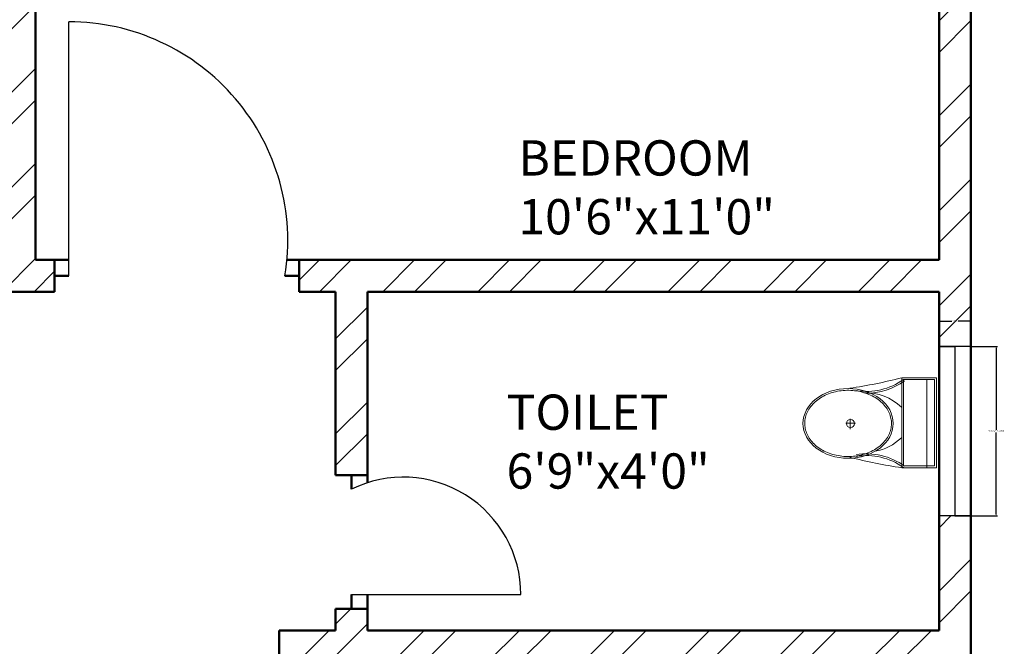
# Model space of a CAD drawing. Units: inches. Extents: x 1901 to 2863, y 888 to 2433.
# Tile 40 of 91: x 2618 to 2758, y 1474 to 1563. Entities that reach past the tile are written whole.
import ezdxf

# ---------------------------------------------------------------- set-up
doc = ezdxf.new("R2010")
doc.units = ezdxf.units.IN
for name, color, linetype, lineweight in [('A-ANNO-DIMS', 2, 'Continuous', 18), ('A-AREA-IDEN', 7, 'Continuous', 18), ('A-DOOR', 4, 'Continuous', 25), ('A-FLOR-FIXT', 9, 'Continuous', 18), ('A-GLAZ', 3, 'Continuous', 25), ('A-WALL', 7, 'Continuous', 50), ('A-WALL-PATT', 8, 'Continuous', 13)]:
    doc.layers.add(name, color=color, linetype=linetype, lineweight=lineweight)
doc.styles.get("Standard").update_dxf_attribs({"font": 'arial.ttf'})
doc.dimstyles.get("Standard").update_dxf_attribs({"dimtxt": 0.18, "dimasz": 0.18, "dimexe": 0.18, "dimexo": 0.0625, "dimgap": 0.09, "dimtad": 0, "dimtih": 1, "dimtoh": 1, "dimdec": 4, "dimzin": 0, "dimdsep": 46, "dimtxsty": 'Standard', "dimcen": 0.09, "dimadec": 0, "dimazin": 0, "dimtfac": 1, "dimtdec": 4, "dimtofl": 0, "dimtmove": 0, "dimatfit": 3, "dimfxl": 1, "dimtolj": 1, "dimtzin": 0, "dimarcsym": 0})

# ---------------------------------------------------------------- blocks, each defined once
blk = doc.blocks.new('A$C31115884')
for p, q in [((257.5, 466.4), (257.5, 523.2)), ((283.1, 497.7), (223.4, 497.7)), ((0, 200), (0, 0)), ((520, 200), (0, 200)), ((10, 190), (10, 10)), ((510, 190), (10, 190)), ((510, 10), (510, 190)), ((520, 0), (520, 200)), ((510, 54.5), (0, 54.5)), ((10, 10), (510, 10)), ((0, 0), (520, 0))]:
    blk.add_line(p, q)
blk.add_circle((255.6, 496.4), 23.6)
for centre, radius, start, end in [((2777.7, -204.6), 2807, 165.4549, 171.7133), ((-294.5, 403.3), 364.7, 324.2091, 9.3499), ((-294.5, 403.3), 374.7, 324.2091, 9.3499), ((805.8, 403.3), 364.7, 170.6501, 215.7909), ((3237, 905), 2807, 188.2867, 194.5451), ((139.5, 406.2), 293.5, 315.8436, 2.6563), ((805.8, 403.3), 374.7, 179.2036, 215.7909), ((383.6, 406.2), 293.5, 190.2774, 224.1564)]:
    blk.add_arc(centre, radius, start, end)
blk.add_ellipse((256.2, 509.9), major_axis=(0, -260.7), ratio=0.772727)
blk.add_open_spline([(256.2, 259.2), (263.1, 259.2), (270, 259.7), (287.8, 262.3), (298.7, 265.1), (319.9, 273.1), (330.2, 278.4), (350.1, 291.1), (359.7, 298.7), (377.7, 315.9), (386.2, 325.5), (401.7, 346.6), (408.8, 358.1), (421.3, 382.5), (426.8, 395.5), (435.9, 422.4), (439.5, 436.4), (444.8, 465.1), (446.5, 479.7), (447.9, 509.2), (447.6, 524), (445, 553.3), (442.7, 567.8), (436.3, 596), (432.1, 609.7), (421.9, 636), (416, 648.6), (402.5, 672.1), (395, 683), (378.6, 703), (369.8, 712.1), (351.1, 728), (341.3, 734.8), (320.9, 746.2), (310.4, 750.7), (288.9, 757.3), (278, 759.4), (256, 761), (245, 760.6), (223.1, 757.2), (212.3, 754.3), (191.1, 746.1), (180.8, 740.7), (160.9, 727.8), (151.4, 720.1), (133.5, 702.7), (125.1, 693), (109.6, 671.7), (102.6, 660.2), (90.2, 635.7), (84.9, 622.7), (76, 595.6), (72.4, 581.6), (67.2, 552.9), (65.6, 538.2), (64.4, 508.8), (64.8, 494), (67.5, 464.7), (69.9, 450.2), (76.6, 422), (80.8, 408.3), (91.1, 382.2), (97.2, 369.7), (110.8, 346.3), (118.4, 335.4), (134.8, 315.6), (143.7, 306.7), (162.4, 290.9), (172.3, 284.2), (192.8, 273), (203.3, 268.6), (224.8, 262.2), (235.8, 260.2), (249.9, 259.3), (253, 259.2), (256.2, 259.2)], degree=3, knots=[0, 0, 0, 0, 0.110105, 0.110105, 0.285049, 0.285049, 0.459994, 0.459994, 0.634938, 0.634938, 0.809882, 0.809882, 0.984827, 0.984827, 1.159771, 1.159771, 1.334715, 1.334715, 1.50966, 1.50966, 1.684604, 1.684604, 1.859549, 1.859549, 2.034493, 2.034493, 2.209437, 2.209437, 2.384382, 2.384382, 2.559326, 2.559326, 2.73427, 2.73427, 2.909215, 2.909215, 3.084159, 3.084159, 3.259103, 3.259103, 3.434048, 3.434048, 3.608992, 3.608992, 3.783936, 3.783936, 3.958881, 3.958881, 4.133825, 4.133825, 4.30877, 4.30877, 4.483714, 4.483714, 4.658658, 4.658658, 4.833603, 4.833603, 5.008547, 5.008547, 5.183491, 5.183491, 5.358436, 5.358436, 5.53338, 5.53338, 5.708324, 5.708324, 5.883269, 5.883269, 6.058213, 6.058213, 6.233158, 6.233158, 6.283185, 6.283185, 6.283185, 6.283185])
blk = doc.blocks.new('WIN-24')
for p, q in [((0, 4.5), (0, 0)), ((24, 2.25), (24, 4.5)), ((24, 4.5), (24, 0)), ((0, 0), (0, 2.25)), ((0, 2.25), (24, 2.25))]:
    blk.add_line(p, q)
blk = doc.blocks.new('*D23')
at = {"layer": 'A-ANNO-DIMS', "color": 0, "lineweight": -2, "transparency": 16777216}
for p, q in [((2752.99, 1516.88), (2756.71, 1516.88)), ((2756.53, 1516.7), (2756.53, 1505.06)), ((2756.53, 1493.06), (2756.53, 1504.7)), ((2752.99, 1492.88), (2756.71, 1492.88))]:
    blk.add_line(p, q, dxfattribs=at)
at = {"layer": 'A-ANNO-DIMS', "color": 0, "transparency": 16777216}
for points in [[(2756.5, 1516.7), (2756.56, 1516.7), (2756.53, 1516.88)], [(2756.5, 1493.06), (2756.56, 1493.06), (2756.53, 1492.88)]]:
    blk.add_solid(points, dxfattribs=at)
at = {"layer": 'Defpoints', "color": 0, "transparency": 16777216}
for p in [(2752.93, 1516.88), (2752.93, 1492.88), (2756.53, 1492.88)]:
    blk.add_point(p, dxfattribs=at)
at = {"layer": 'A-ANNO-DIMS', "color": 0, "transparency": 16777216, "insert": (2756.53, 1504.88), "char_height": 0.18, "attachment_point": 5}
blk.add_mtext('\\A1;WINDOW W3 24 TYP.', dxfattribs=at)
blk = doc.blocks.new('*D24')
at = {"layer": 'A-ANNO-DIMS', "color": 0, "lineweight": -2, "transparency": 16777216}
for p, q in [((2748.43, 1516.94), (2748.43, 1520.66)), ((2748.61, 1520.48), (2750.22, 1520.48)), ((2752.75, 1520.48), (2751.13, 1520.48)), ((2752.93, 1516.94), (2752.93, 1520.66))]:
    blk.add_line(p, q, dxfattribs=at)
at = {"layer": 'A-ANNO-DIMS', "color": 0, "transparency": 16777216}
for points in [[(2748.61, 1520.51), (2748.61, 1520.45), (2748.43, 1520.48)], [(2752.75, 1520.51), (2752.75, 1520.45), (2752.93, 1520.48)]]:
    blk.add_solid(points, dxfattribs=at)
at = {"layer": 'Defpoints', "color": 0, "transparency": 16777216}
for p in [(2752.93, 1520.48), (2748.43, 1516.88), (2752.93, 1516.88)]:
    blk.add_point(p, dxfattribs=at)
at = {"layer": 'A-ANNO-DIMS', "color": 0, "transparency": 16777216, "insert": (2750.68, 1520.48), "char_height": 0.18, "attachment_point": 5}
blk.add_mtext('\\A1;5 TYP.', dxfattribs=at)

msp = doc.modelspace()

# ---------------------------------------------------------------- hatches: boundary and pattern name
at = {"layer": 'A-WALL-PATT'}
h = msp.add_hatch(dxfattribs=at)
h.set_pattern_fill('ANSI32', color=256)
h.paths.add_polyline_path([(2192.5, 2274.13), (2141.26, 2274.13), (2141.26, 2269.63), (2192.5, 2269.63)])
h.paths.add_polyline_path([(2259.93, 2274.13), (2216.5, 2274.13), (2216.5, 2269.63), (2255.43, 2269.63), (2255.43, 2214.63), (2250.81, 2214.63), (2250.81, 2210.13), (2259.93, 2210.13), (2259.93, 2215.13), (2271.76, 2215.13), (2271.76, 2217.38), (2271.76, 2219.63), (2259.93, 2219.63)])
h.paths.add_polyline_path([(2171.43, 2269.63), (2166.93, 2269.63), (2166.93, 2219.63), (2121.24, 2219.63), (2121.24, 2215.13), (2166.93, 2215.13), (2166.93, 2083.13), (2161.81, 2083.13), (2161.81, 2078.63), (2171.43, 2078.63), (2177, 2078.63), (2177, 2080.88), (2177, 2083.13), (2171.43, 2083.13), (2171.43, 2210.13), (2230.91, 2210.13), (2230.91, 2212.38), (2230.91, 2214.63), (2171.43, 2214.63)])
h.paths.add_polyline_path([(2117.26, 2274.13), (2089.43, 2274.13), (2089.43, 2219.63), (2081.14, 2219.63), (2081.14, 2215.13), (2089.43, 2215.13), (2098, 2215.13), (2098, 2217.38), (2098, 2219.63), (2093.93, 2219.63), (2093.93, 2269.63), (2117.26, 2269.63), (2117.26, 2271.88)])
h.paths.add_polyline_path([(2343.43, 2219.63), (2329.29, 2219.63), (2329.29, 2215.13), (2338.93, 2215.13), (2338.93, 2184.74), (2343.43, 2184.74)])
h.paths.add_polyline_path([(2338.93, 2083.13), (2329.29, 2083.13), (2208.97, 2083.13), (2208.97, 2078.63), (2338.93, 2078.63)])
h.paths.add_polyline_path([(2343.43, 2136.74), (2338.93, 2136.74), (2338.93, 1872.63), (2343.43, 1872.63)])
h.paths.add_polyline_path([(2343.43, 1863.63), (2397.68, 1863.63), (2397.68, 1821.63), (2384.14, 1821.63), (2384.14, 1812.63), (2418.33, 1812.63), (2418.33, 1817.13), (2418.33, 1821.63), (2406.68, 1821.63), (2406.68, 1863.63), (2459.5, 1863.63), (2459.5, 1821.63), (2447.14, 1821.63), (2447.14, 1812.63), (2459.5, 1812.63), (2468.5, 1812.63), (2468.5, 1872.63), (2394.43, 1872.63), (2334.43, 1872.63), (2334.43, 1812.63), (2343.43, 1812.63), (2353.25, 1812.63), (2353.25, 1821.63), (2343.43, 1821.63)])
h.paths.add_polyline_path([(2510.01, 1872.63), (2468.5, 1872.63), (2468.5, 1868.13), (2510.01, 1868.13)])
h.paths.add_polyline_path([(2514.01, 1817.13), (2468.5, 1817.13), (2468.5, 1812.63), (2482.11, 1812.63), (2482.11, 1800.61), (2486.61, 1800.61), (2486.61, 1812.63), (2514.01, 1812.63)])
h.paths.add_polyline_path([(2299.25, 1814.88), (2299.25, 1817.13), (2295.93, 1817.13), (2295.93, 1854.17), (2293.68, 1854.17), (2291.43, 1854.17), (2291.43, 1817.13), (2266.11, 1817.13), (2266.11, 1812.63), (2299.25, 1812.63)])
h.paths.add_polyline_path([(2218.11, 1817.13), (2206.46, 1817.13), (2171.43, 1817.13), (2171.43, 1949.13), (2190.1, 1949.13), (2190.1, 1953.63), (2163.47, 1953.63), (2163.47, 1949.13), (2166.93, 1949.13), (2166.93, 1817.13), (2114.3, 1817.13), (2114.3, 1812.63), (2218.11, 1812.63)])
h.paths.add_polyline_path([(2029.43, 1970.92), (2024.93, 1970.92), (2024.93, 1912.72), (2029.43, 1912.72)])
h.paths.add_polyline_path([(2132.3, 1953.63), (2113.93, 1953.63), (2113.93, 1975.89), (2111.68, 1975.89), (2109.43, 1975.89), (2109.43, 1953.63), (2029.43, 1953.63), (2029.43, 1949.13), (2132.3, 1949.13)])
h.paths.add_polyline_path([(2029.43, 1853.61), (2029.31, 1853.61), (2029.31, 1853.61), (2029.43, 1853.61), (2029.43, 1864.72), (2024.93, 1864.72), (2024.93, 1812.63), (2066.3, 1812.63), (2066.3, 1814.88), (2066.3, 1817.13), (2029.43, 1817.13)])
h.paths.add_polyline_path([(2122.93, 2010.09), (2120.68, 2010.09), (2118.43, 2010.09), (2118.43, 2006.13), (2029.43, 2006.13), (2029.43, 2001.63), (2109.43, 2001.63), (2109.43, 1998.04), (2113.93, 1998.04), (2113.93, 2001.63), (2122.93, 2001.63)])
h.paths.add_polyline_path([(2029.43, 2031.38), (2024.93, 2031.38), (2024.93, 1994.92), (2027.18, 1994.92), (2029.43, 1994.92)])
h.paths.add_polyline_path([(2029.43, 2136.74), (2024.93, 2136.74), (2024.93, 2067.38), (2027.18, 2067.38), (2029.43, 2067.38)])
h.paths.add_polyline_path([(2125.62, 2083.13), (2029.43, 2083.13), (2029.43, 2078.63), (2118.43, 2078.63), (2118.43, 2030.71), (2122.93, 2030.71), (2122.93, 2078.63), (2125.62, 2078.63)])
h.paths.add_polyline_path([(2029.43, 2215.13), (2040.47, 2215.13), (2040.47, 2217.38), (2040.47, 2219.63), (2024.93, 2219.63), (2024.93, 2184.74), (2029.43, 2184.74), (2029.43, 2187.78)])
h.paths.add_polyline_path([(2686.43, 2274.13), (2659.28, 2274.13), (2659.28, 2269.63), (2681.93, 2269.63), (2681.93, 2219.63), (2676.82, 2219.63), (2676.82, 2215.13), (2681.93, 2215.13), (2697.01, 2215.13), (2697.01, 2217.38), (2697.01, 2219.63), (2686.43, 2219.63)])
h.paths.add_polyline_path([(2609.93, 2269.63), (2635.28, 2269.63), (2635.28, 2274.13), (2571.43, 2274.13), (2571.43, 2269.63), (2605.43, 2269.63), (2605.43, 2214.63), (2549.1, 2214.63), (2549.1, 2210.13), (2605.43, 2210.13), (2605.43, 2083.13), (2601.01, 2083.13), (2601.01, 2080.88), (2601.01, 2078.63), (2609.93, 2078.63), (2616.16, 2078.63), (2616.16, 2080.88), (2616.16, 2083.13), (2609.93, 2083.13), (2609.93, 2215.13), (2651.46, 2215.13), (2651.46, 2217.38), (2651.46, 2219.63), (2609.93, 2219.63)])
h.paths.add_polyline_path([(2521.43, 2269.63), (2547.43, 2269.63), (2547.43, 2271.88), (2547.43, 2274.13), (2516.93, 2274.13), (2516.93, 2219.63), (2506.41, 2219.63), (2506.41, 2215.13), (2516.93, 2215.13), (2516.93, 2210.13), (2525.4, 2210.13), (2525.4, 2212.38), (2525.4, 2214.63), (2521.43, 2214.63)])
h.paths.add_polyline_path([(2456.01, 2219.63), (2439.43, 2219.63), (2439.43, 2187.89), (2443.93, 2187.89), (2443.93, 2215.13), (2456.01, 2215.13)])
h.paths.add_polyline_path([(2752.93, 2219.63), (2739.48, 2219.63), (2739.48, 2215.13), (2748.43, 2215.13), (2748.43, 2187.89), (2752.93, 2187.89)])
h.paths.add_polyline_path([(2752.93, 2139.89), (2748.43, 2139.89), (2748.43, 2083.13), (2648.42, 2083.13), (2648.42, 2078.63), (2654.93, 2078.63), (2654.93, 2039.44), (2659.43, 2039.44), (2659.43, 2078.63), (2748.43, 2078.63), (2748.43, 2063.43), (2752.93, 2063.43)])
h.paths.add_polyline_path([(2752.93, 2010.63), (2659.43, 2010.63), (2659.43, 2015.65), (2654.93, 2015.65), (2654.93, 2010.63), (2605.43, 2010.63), (2605.43, 1920.97), (2609.93, 1920.97), (2609.93, 2006.13), (2748.43, 2006.13), (2748.43, 1982.47), (2752.93, 1982.47)])
h.paths.add_polyline_path([(2752.93, 2027.43), (2748.43, 2027.43), (2748.43, 2010.63), (2752.93, 2010.63)])
h.paths.add_polyline_path([(2748.43, 1886.13), (2609.93, 1886.13), (2609.93, 1889.72), (2605.43, 1889.72), (2605.43, 1861.26), (2609.93, 1861.26), (2609.93, 1881.63), (2748.43, 1881.63)])
h.paths.add_polyline_path([(2456.86, 2228.83), (2498.4, 2228.83), (2498.4, 2247.49), (2456.86, 2247.49)], flags=9)
h.paths.add_polyline_path([(2038.6, 2237.42), (2080.17, 2237.42), (2080.17, 2256.08), (2038.6, 2256.08)], flags=9)
h.paths.add_polyline_path([(2292.01, 1062.39), (2539.93, 1062.39), (2539.93, 1099.49), (2292.01, 1099.49)], flags=9)
h.paths.add_polyline_path([(2424.91, 1832.25), (2448.51, 1832.25), (2448.51, 1846.68), (2424.91, 1846.68)], flags=25)
h.paths.add_polyline_path([(2359.08, 1832.25), (2382.68, 1832.25), (2382.68, 1846.68), (2359.08, 1846.68)], flags=25)
h.paths.add_polyline_path([(2352.9, 1684.8), (2367.54, 1684.8), (2367.54, 1697.17), (2352.9, 1697.17)], flags=9)
h.paths.add_polyline_path([(2079.29, 1755.83), (2169.02, 1755.83), (2169.02, 1774.37), (2079.29, 1774.37)], flags=9)
h.paths.add_polyline_path([(2404.09, 1373.86), (2404.09, 1463.59), (2385.54, 1463.59), (2385.54, 1373.86)], flags=9)
h.paths.add_polyline_path([(2268.09, 2236.37), (2309.64, 2236.37), (2309.64, 2255.03), (2268.09, 2255.03)], flags=9)
h.paths.add_polyline_path([(2575.96, 1700.95), (2665.7, 1700.95), (2665.7, 1719.5), (2575.96, 1719.5)], flags=9)
h.paths.add_polyline_path([(2302.96, 1878.47), (2329.52, 1878.47), (2329.52, 1888.78), (2302.96, 1888.78)], flags=9)
h.paths.add_polyline_path([(2097.42, 2240.58), (2126.57, 2240.58), (2126.57, 2259.23), (2097.42, 2259.23)], flags=9)
h.paths.add_polyline_path([(2208.72, 2246.12), (2237.88, 2246.12), (2237.88, 2264.78), (2208.72, 2264.78)], flags=9)
h.paths.add_polyline_path([(2038.15, 1925.96), (2076.99, 1925.96), (2076.99, 1944.62), (2038.15, 1944.62)], flags=9)
h.paths.add_polyline_path([(2239.14, 1926.67), (2288.46, 1926.67), (2288.46, 1945.33), (2239.14, 1945.33)], flags=9)
h.paths.add_polyline_path([(2175.43, 2007.33), (2212.36, 2007.33), (2212.36, 2025.99), (2175.43, 2025.99)], flags=9)
h.paths.add_polyline_path([(2225.03, 2091.79), (2263.87, 2091.79), (2263.87, 2110.45), (2225.03, 2110.45)], flags=9)
h.paths.add_polyline_path([(2035.4, 2098.48), (2074.24, 2098.48), (2074.24, 2117.14), (2035.4, 2117.14)], flags=9)
h.paths.add_polyline_path([(2050.1, 2029.21), (2083.26, 2029.21), (2083.26, 2047.87), (2050.1, 2047.87)], flags=9)
h.paths.add_polyline_path([(2069.68, 1956.72), (2098.83, 1956.72), (2098.83, 1975.38), (2069.68, 1975.38)], flags=25)
h.paths.add_polyline_path([(2328.62, 1753.34), (2361.66, 1753.34), (2361.66, 1771.99), (2328.62, 1771.99)], flags=9)
h.paths.add_polyline_path([(2395.16, 2060.89), (2395.16, 2140.65), (2378.68, 2140.65), (2378.68, 2060.89)], flags=9)
h.paths.add_polyline_path([(2463.73, 2059.02), (2492.89, 2059.02), (2492.89, 2077.68), (2463.73, 2077.68)], flags=9)
h.paths.add_polyline_path([(2458.03, 2181.54), (2496.87, 2181.54), (2496.87, 2200.19), (2458.03, 2200.19)], flags=9)
h.paths.add_polyline_path([(2527.58, 2243.07), (2556.73, 2243.07), (2556.73, 2261.73), (2527.58, 2261.73)], flags=9)
h.paths.add_polyline_path([(2694.46, 2232.77), (2736.03, 2232.77), (2736.03, 2251.42), (2694.46, 2251.42)], flags=9)
h.paths.add_polyline_path([(2637.82, 2249.22), (2666.98, 2249.22), (2666.98, 2267.88), (2637.82, 2267.88)], flags=9)
h.paths.add_polyline_path([(2623.69, 2183.54), (2662.53, 2183.54), (2662.53, 2202.2), (2623.69, 2202.2)], flags=9)
h.paths.add_polyline_path([(2691.97, 2021.5), (2725.12, 2021.5), (2725.12, 2040.16), (2691.97, 2040.16)], flags=9)
h.paths.add_polyline_path([(2621.04, 1975.91), (2662.34, 1975.91), (2662.34, 1994.57), (2621.04, 1994.57)], flags=25)
h.paths.add_polyline_path([(2479.03, 1927.62), (2519.84, 1927.62), (2519.84, 1946.28), (2479.03, 1946.28)], flags=9)
h.paths.add_polyline_path([(2670.94, 1849.08), (2716.01, 1849.08), (2716.01, 1867.73), (2670.94, 1867.73)], flags=9)
h.paths.add_polyline_path([(2523.61, 1782.96), (2550.17, 1782.96), (2550.17, 1793.26), (2523.61, 1793.26)], flags=9)
h.paths.add_polyline_path([(2450.84, 1207.33), (2492.39, 1207.33), (2492.39, 1225.99), (2450.84, 1225.99)], flags=9)
h.paths.add_polyline_path([(2527.75, 1203.84), (2556.91, 1203.84), (2556.91, 1222.5), (2527.75, 1222.5)], flags=9)
h.paths.add_polyline_path([(2639.11, 1207.2), (2668.27, 1207.2), (2668.27, 1225.86), (2639.11, 1225.86)], flags=9)
h.paths.add_polyline_path([(2692.59, 1218.97), (2734.17, 1218.97), (2734.17, 1237.62), (2692.59, 1237.62)], flags=9)
h.paths.add_polyline_path([(2669.27, 1366.33), (2708.11, 1366.33), (2708.11, 1384.99), (2669.27, 1384.99)], flags=9)
h.paths.add_polyline_path([(2463.31, 1358.03), (2502.15, 1358.03), (2502.15, 1376.69), (2463.31, 1376.69)], flags=9)
h.paths.add_polyline_path([(2494.72, 1449.96), (2531.65, 1449.96), (2531.65, 1468.62), (2494.72, 1468.62)], flags=9)
h.paths.add_polyline_path([(2675.57, 1422.16), (2708.72, 1422.16), (2708.72, 1440.81), (2675.57, 1440.81)], flags=9)
h.paths.add_polyline_path([(2685.63, 1493.89), (2714.79, 1493.89), (2714.79, 1512.55), (2685.63, 1512.55)], flags=9)
h.paths.add_polyline_path([(2686.8, 1529.91), (2725.65, 1529.91), (2725.65, 1548.57), (2686.8, 1548.57)], flags=9)
h.paths.add_polyline_path([(2503.65, 1537.99), (2552.97, 1537.99), (2552.97, 1556.65), (2503.65, 1556.65)], flags=9)
h.paths.add_polyline_path([(2291.71, 1643.5), (2318.28, 1643.5), (2318.28, 1653.81), (2291.71, 1653.81)], flags=9)
h.paths.add_polyline_path([(2450.63, 1610.52), (2477.19, 1610.52), (2477.19, 1620.82), (2450.63, 1620.82)], flags=9)
h.paths.add_polyline_path([(2359.99, 1551.81), (2422.25, 1551.81), (2422.25, 1562.12), (2359.99, 1562.12)], flags=9)
h.paths.add_polyline_path([(2280.11, 1249.01), (2321.65, 1249.01), (2321.65, 1267.66), (2280.11, 1267.66)], flags=9)
h.paths.add_polyline_path([(2164.06, 1274.23), (2193.22, 1274.23), (2193.22, 1292.89), (2164.06, 1292.89)], flags=9)
h.paths.add_polyline_path([(2118.21, 1277.69), (2151.25, 1277.69), (2151.25, 1296.35), (2118.21, 1296.35)], flags=9)
h.paths.add_polyline_path([(2031.95, 1268.53), (2073.52, 1268.53), (2073.52, 1287.19), (2031.95, 1287.19)], flags=9)
h.paths.add_polyline_path([(2050.2, 1409.08), (2089.04, 1409.08), (2089.04, 1427.74), (2050.2, 1427.74)], flags=9)
h.paths.add_polyline_path([(2243.74, 1421.03), (2282.58, 1421.03), (2282.58, 1439.69), (2243.74, 1439.69)], flags=9)
h.paths.add_polyline_path([(2190.75, 1509.77), (2231.56, 1509.77), (2231.56, 1528.43), (2190.75, 1528.43)], flags=9)
h.paths.add_polyline_path([(2058.39, 1475.42), (2091.55, 1475.42), (2091.55, 1494.07), (2058.39, 1494.07)], flags=9)
h.paths.add_polyline_path([(2062.45, 1553.09), (2091.6, 1553.09), (2091.6, 1571.75), (2062.45, 1571.75)], flags=9)
h.paths.add_polyline_path([(2219.52, 1590.37), (2266.15, 1590.37), (2266.15, 1609.02), (2219.52, 1609.02)], flags=9)
h.paths.add_polyline_path([(2041.07, 1584.19), (2079.91, 1584.19), (2079.91, 1602.85), (2041.07, 1602.85)], flags=9)
h = msp.add_hatch(dxfattribs=at)
h.set_pattern_fill('ANSI32', color=256)
h.paths.add_polyline_path([(2443.93, 2139.89), (2439.43, 2139.89), (2439.43, 2069.35), (2441.68, 2069.35), (2443.93, 2069.35), (2443.93, 2078.63), (2521.93, 2078.63), (2521.93, 2075.07), (2524.18, 2075.07), (2526.43, 2075.07), (2526.43, 2078.63), (2571.75, 2078.63), (2571.75, 2080.88), (2571.75, 2083.13), (2443.93, 2083.13)])
h.paths.add_polyline_path([(2526.43, 2054.63), (2524.18, 2054.63), (2521.93, 2054.63), (2521.93, 2030.63), (2443.93, 2030.63), (2443.93, 2045.35), (2439.43, 2045.35), (2439.43, 1983.87), (2443.93, 1983.87), (2443.93, 2026.13), (2521.93, 2026.13), (2526.43, 2026.13)])
h.paths.add_polyline_path([(2443.93, 1923.87), (2439.43, 1923.87), (2439.43, 1872.63), (2443.93, 1872.63)])
h.paths.add_polyline_path([(2636.23, 1766.13), (2609.93, 1766.13), (2609.93, 1779.79), (2605.43, 1779.79), (2605.43, 1766.13), (2486.61, 1766.13), (2486.61, 1770.67), (2482.11, 1770.67), (2482.11, 1766.13), (2482.11, 1761.63), (2636.23, 1761.63), (2636.23, 1763.88)])
h.paths.add_polyline_path([(2519.54, 1663.38), (2519.54, 1665.63), (2494.93, 1665.63), (2481.83, 1665.63), (2481.83, 1663.38), (2481.83, 1661.13), (2490.43, 1661.13), (2490.43, 1640.16), (2494.93, 1640.16), (2494.93, 1661.13), (2519.54, 1661.13)])
h.paths.add_polyline_path([(2443.93, 1712.13), (2443.93, 1716.63), (2414.46, 1716.63), (2414.46, 1712.13), (2439.43, 1712.13), (2439.43, 1545.51), (2443.93, 1545.51), (2443.93, 1661.13), (2448.47, 1661.13), (2448.47, 1665.63), (2443.93, 1665.63)])
h.paths.add_polyline_path([(2343.43, 1712.13), (2365.52, 1712.13), (2365.52, 1714.38), (2365.52, 1716.63), (2333.87, 1716.63), (2333.87, 1714.38), (2333.87, 1712.13), (2338.93, 1712.13), (2338.93, 1575.63), (2338.93, 1545.51), (2343.43, 1545.51), (2343.43, 1547.51), (2343.43, 1580.13)])
h.paths.add_polyline_path([(2752.93, 1665.63), (2579.54, 1665.63), (2579.54, 1661.13), (2615.93, 1661.13), (2615.93, 1529.13), (2598.93, 1529.13), (2598.93, 1524.63), (2623.13, 1524.63), (2623.13, 1526.88), (2623.13, 1529.13), (2620.43, 1529.13), (2620.43, 1661.13), (2748.43, 1661.13), (2748.43, 1633.5), (2752.93, 1633.5)])
h.paths.add_polyline_path([(2752.93, 1419.93), (2748.43, 1419.93), (2748.43, 1400.13), (2659.43, 1400.13), (2659.43, 1444.33), (2657.18, 1444.33), (2654.93, 1444.33), (2654.93, 1400.13), (2643.65, 1400.13), (2643.65, 1395.63), (2748.43, 1395.63), (2748.43, 1364.04), (2752.93, 1364.04)])
h.paths.add_polyline_path([(2752.93, 1492.88), (2748.43, 1492.88), (2748.43, 1476.63), (2667.43, 1476.63), (2667.43, 1479.71), (2665.18, 1479.71), (2662.93, 1479.71), (2662.93, 1476.63), (2654.93, 1476.63), (2654.93, 1469.54), (2659.43, 1469.54), (2659.43, 1472.13), (2748.43, 1472.13), (2748.43, 1455.93), (2752.93, 1455.93)])
h.paths.add_polyline_path([(2752.93, 1304.04), (2748.43, 1304.04), (2748.43, 1263.63), (2738.66, 1263.63), (2738.66, 1259.13), (2752.93, 1259.13)])
h.paths.add_polyline_path([(2685.93, 1259.13), (2695.49, 1259.13), (2695.49, 1261.38), (2695.49, 1263.63), (2677.84, 1263.63), (2677.84, 1261.38), (2677.84, 1259.13), (2681.43, 1259.13), (2681.43, 1203.63), (2653.28, 1203.63), (2653.28, 1199.13), (2685.93, 1199.13), (2685.93, 1203.63)])
h.paths.add_polyline_path([(2609.43, 1395.63), (2611.85, 1395.63), (2611.85, 1400.13), (2598.89, 1400.13), (2598.89, 1397.88), (2598.89, 1395.63), (2604.93, 1395.63), (2604.93, 1268.13), (2554.73, 1268.13), (2554.73, 1265.88), (2554.73, 1263.63), (2604.93, 1263.63), (2604.93, 1203.63), (2571.31, 1203.63), (2571.31, 1199.13), (2604.93, 1199.13), (2629.28, 1199.13), (2629.28, 1201.38), (2629.28, 1203.63), (2609.43, 1203.63), (2609.43, 1258.63), (2609.43, 1259.13), (2654.8, 1259.13), (2654.8, 1263.63), (2609.43, 1263.63)])
h.paths.add_polyline_path([(2443.93, 1304.04), (2439.43, 1304.04), (2439.43, 1259.13), (2443.93, 1259.13), (2456.16, 1259.13), (2456.16, 1261.38), (2456.16, 1263.63), (2443.93, 1263.63)])
h.paths.add_polyline_path([(2525.43, 1263.63), (2531.78, 1263.63), (2531.78, 1268.13), (2520.93, 1268.13), (2520.93, 1263.63), (2511.41, 1263.63), (2511.41, 1259.13), (2520.93, 1259.13), (2520.93, 1199.13), (2547.31, 1199.13), (2547.31, 1201.38), (2547.31, 1203.63), (2525.43, 1203.63)])
h.paths.add_polyline_path([(2443.93, 1434.84), (2439.43, 1434.84), (2439.43, 1364.04), (2441.68, 1364.04), (2443.93, 1364.04)])
h.paths.add_polyline_path([(2567.13, 1400.13), (2443.93, 1400.13), (2443.93, 1395.63), (2567.13, 1395.63)])
h.paths.add_polyline_path([(2443.93, 1545.51), (2439.43, 1545.51), (2439.43, 1494.84), (2443.93, 1494.84)])
h.paths.add_polyline_path([(2494.93, 1553.35), (2492.68, 1553.35), (2490.43, 1553.35), (2490.43, 1524.63), (2494.93, 1524.63), (2525.94, 1524.63), (2525.94, 1526.88), (2525.94, 1529.13), (2494.93, 1529.13)])
h.paths.add_polyline_path([(2752.93, 1573.5), (2748.43, 1573.5), (2748.43, 1529.13), (2657.76, 1529.13), (2657.76, 1524.63), (2662.93, 1524.63), (2662.93, 1498.63), (2667.43, 1498.63), (2667.43, 1524.63), (2748.43, 1524.63), (2748.43, 1516.88), (2752.93, 1516.88)])
h.paths.add_polyline_path([(2038.6, 2237.42), (2080.17, 2237.42), (2080.17, 2256.08), (2038.6, 2256.08)], flags=9)
h.paths.add_polyline_path([(2292.01, 1062.39), (2539.93, 1062.39), (2539.93, 1099.49), (2292.01, 1099.49)], flags=9)
h.paths.add_polyline_path([(2424.91, 1832.25), (2448.51, 1832.25), (2448.51, 1846.68), (2424.91, 1846.68)], flags=9)
h.paths.add_polyline_path([(2359.08, 1832.25), (2382.68, 1832.25), (2382.68, 1846.68), (2359.08, 1846.68)], flags=9)
h.paths.add_polyline_path([(2352.9, 1684.8), (2367.54, 1684.8), (2367.54, 1697.17), (2352.9, 1697.17)], flags=9)
h.paths.add_polyline_path([(2079.29, 1755.83), (2169.02, 1755.83), (2169.02, 1774.37), (2079.29, 1774.37)], flags=9)
h.paths.add_polyline_path([(2404.09, 1373.86), (2404.09, 1463.59), (2385.54, 1463.59), (2385.54, 1373.86)], flags=9)
h.paths.add_polyline_path([(2268.09, 2236.37), (2309.64, 2236.37), (2309.64, 2255.03), (2268.09, 2255.03)], flags=9)
h.paths.add_polyline_path([(2575.96, 1700.95), (2665.7, 1700.95), (2665.7, 1719.5), (2575.96, 1719.5)], flags=9)
h.paths.add_polyline_path([(2302.96, 1878.47), (2329.52, 1878.47), (2329.52, 1888.78), (2302.96, 1888.78)], flags=9)
h.paths.add_polyline_path([(2097.42, 2240.58), (2126.57, 2240.58), (2126.57, 2259.23), (2097.42, 2259.23)], flags=9)
h.paths.add_polyline_path([(2208.72, 2246.12), (2237.88, 2246.12), (2237.88, 2264.78), (2208.72, 2264.78)], flags=9)
h.paths.add_polyline_path([(2038.15, 1925.96), (2076.99, 1925.96), (2076.99, 1944.62), (2038.15, 1944.62)], flags=9)
h.paths.add_polyline_path([(2239.14, 1926.67), (2288.46, 1926.67), (2288.46, 1945.33), (2239.14, 1945.33)], flags=9)
h.paths.add_polyline_path([(2175.43, 2007.33), (2212.36, 2007.33), (2212.36, 2025.99), (2175.43, 2025.99)], flags=9)
h.paths.add_polyline_path([(2225.03, 2091.79), (2263.87, 2091.79), (2263.87, 2110.45), (2225.03, 2110.45)], flags=9)
h.paths.add_polyline_path([(2035.4, 2098.48), (2074.24, 2098.48), (2074.24, 2117.14), (2035.4, 2117.14)], flags=9)
h.paths.add_polyline_path([(2050.1, 2029.21), (2083.26, 2029.21), (2083.26, 2047.87), (2050.1, 2047.87)], flags=9)
h.paths.add_polyline_path([(2069.68, 1956.72), (2098.83, 1956.72), (2098.83, 1975.38), (2069.68, 1975.38)], flags=9)
h.paths.add_polyline_path([(2328.62, 1753.34), (2361.66, 1753.34), (2361.66, 1771.99), (2328.62, 1771.99)], flags=9)
h.paths.add_polyline_path([(2395.16, 2060.89), (2395.16, 2140.65), (2378.68, 2140.65), (2378.68, 2060.89)], flags=9)
h.paths.add_polyline_path([(2463.73, 2059.02), (2492.89, 2059.02), (2492.89, 2077.68), (2463.73, 2077.68)], flags=9)
h.paths.add_polyline_path([(2458.03, 2181.54), (2496.87, 2181.54), (2496.87, 2200.19), (2458.03, 2200.19)], flags=9)
h.paths.add_polyline_path([(2456.86, 2228.83), (2498.4, 2228.83), (2498.4, 2247.49), (2456.86, 2247.49)], flags=9)
h.paths.add_polyline_path([(2527.58, 2243.07), (2556.73, 2243.07), (2556.73, 2261.73), (2527.58, 2261.73)], flags=9)
h.paths.add_polyline_path([(2694.46, 2232.77), (2736.03, 2232.77), (2736.03, 2251.42), (2694.46, 2251.42)], flags=9)
h.paths.add_polyline_path([(2637.82, 2249.22), (2666.98, 2249.22), (2666.98, 2267.88), (2637.82, 2267.88)], flags=9)
h.paths.add_polyline_path([(2623.69, 2183.54), (2662.53, 2183.54), (2662.53, 2202.2), (2623.69, 2202.2)], flags=9)
h.paths.add_polyline_path([(2691.97, 2021.5), (2725.12, 2021.5), (2725.12, 2040.16), (2691.97, 2040.16)], flags=9)
h.paths.add_polyline_path([(2621.04, 1975.91), (2662.34, 1975.91), (2662.34, 1994.57), (2621.04, 1994.57)], flags=9)
h.paths.add_polyline_path([(2479.03, 1927.62), (2519.84, 1927.62), (2519.84, 1946.28), (2479.03, 1946.28)], flags=9)
h.paths.add_polyline_path([(2670.94, 1849.08), (2716.01, 1849.08), (2716.01, 1867.73), (2670.94, 1867.73)], flags=9)
h.paths.add_polyline_path([(2523.61, 1782.96), (2550.17, 1782.96), (2550.17, 1793.26), (2523.61, 1793.26)], flags=9)
h.paths.add_polyline_path([(2450.84, 1207.33), (2492.39, 1207.33), (2492.39, 1225.99), (2450.84, 1225.99)], flags=9)
h.paths.add_polyline_path([(2527.75, 1203.84), (2556.91, 1203.84), (2556.91, 1222.5), (2527.75, 1222.5)], flags=9)
h.paths.add_polyline_path([(2639.11, 1207.2), (2668.27, 1207.2), (2668.27, 1225.86), (2639.11, 1225.86)], flags=9)
h.paths.add_polyline_path([(2692.59, 1218.97), (2734.17, 1218.97), (2734.17, 1237.62), (2692.59, 1237.62)], flags=9)
h.paths.add_polyline_path([(2669.27, 1366.33), (2708.11, 1366.33), (2708.11, 1384.99), (2669.27, 1384.99)], flags=25)
h.paths.add_polyline_path([(2463.31, 1358.03), (2502.15, 1358.03), (2502.15, 1376.69), (2463.31, 1376.69)], flags=9)
h.paths.add_polyline_path([(2494.72, 1449.96), (2531.65, 1449.96), (2531.65, 1468.62), (2494.72, 1468.62)], flags=9)
h.paths.add_polyline_path([(2675.57, 1422.16), (2708.72, 1422.16), (2708.72, 1440.81), (2675.57, 1440.81)], flags=25)
h.paths.add_polyline_path([(2685.63, 1493.89), (2714.79, 1493.89), (2714.79, 1512.55), (2685.63, 1512.55)], flags=9)
h.paths.add_polyline_path([(2686.8, 1529.91), (2725.65, 1529.91), (2725.65, 1548.57), (2686.8, 1548.57)], flags=25)
h.paths.add_polyline_path([(2503.65, 1537.99), (2552.97, 1537.99), (2552.97, 1556.65), (2503.65, 1556.65)], flags=9)
h.paths.add_polyline_path([(2291.71, 1643.5), (2318.28, 1643.5), (2318.28, 1653.81), (2291.71, 1653.81)], flags=9)
h.paths.add_polyline_path([(2450.63, 1610.52), (2477.19, 1610.52), (2477.19, 1620.82), (2450.63, 1620.82)], flags=9)
h.paths.add_polyline_path([(2359.99, 1551.81), (2422.25, 1551.81), (2422.25, 1562.12), (2359.99, 1562.12)], flags=9)
h.paths.add_polyline_path([(2280.11, 1249.01), (2321.65, 1249.01), (2321.65, 1267.66), (2280.11, 1267.66)], flags=9)
h.paths.add_polyline_path([(2164.06, 1274.23), (2193.22, 1274.23), (2193.22, 1292.89), (2164.06, 1292.89)], flags=9)
h.paths.add_polyline_path([(2118.21, 1277.69), (2151.25, 1277.69), (2151.25, 1296.35), (2118.21, 1296.35)], flags=9)
h.paths.add_polyline_path([(2031.95, 1268.53), (2073.52, 1268.53), (2073.52, 1287.19), (2031.95, 1287.19)], flags=9)
h.paths.add_polyline_path([(2050.2, 1409.08), (2089.04, 1409.08), (2089.04, 1427.74), (2050.2, 1427.74)], flags=9)
h.paths.add_polyline_path([(2243.74, 1421.03), (2282.58, 1421.03), (2282.58, 1439.69), (2243.74, 1439.69)], flags=9)
h.paths.add_polyline_path([(2190.75, 1509.77), (2231.56, 1509.77), (2231.56, 1528.43), (2190.75, 1528.43)], flags=9)
h.paths.add_polyline_path([(2058.39, 1475.42), (2091.55, 1475.42), (2091.55, 1494.07), (2058.39, 1494.07)], flags=9)
h.paths.add_polyline_path([(2062.45, 1553.09), (2091.6, 1553.09), (2091.6, 1571.75), (2062.45, 1571.75)], flags=9)
h.paths.add_polyline_path([(2219.52, 1590.37), (2266.15, 1590.37), (2266.15, 1609.02), (2219.52, 1609.02)], flags=9)
h.paths.add_polyline_path([(2041.07, 1584.19), (2079.91, 1584.19), (2079.91, 1602.85), (2041.07, 1602.85)], flags=9)

# ---------------------------------------------------------------- linework, layer by layer
at = {"layer": 'A-DOOR'}
for p, q in [((2625.13, 1526.88), (2625.13, 1562.88)), ((2665.18, 1481.71), (2689.18, 1481.71))]:
    msp.add_line(p, q, dxfattribs=at)
for centre, radius, start, end in [((2625.13, 1531.85), 31.03, 350.7892, 90), ((2672.54, 1481.71), 16.64, 0, 116.2588)]:
    msp.add_arc(centre, radius, start, end, dxfattribs=at)
at = {"layer": 'A-WALL'}
for p, q in [((2752.93, 1665.63), (2752.93, 1259.13)), ((2620.43, 1661.13), (2620.43, 1529.13)), ((2748.43, 1661.13), (2748.43, 1529.13)), ((2620.43, 1529.13), (2625.13, 1529.13)), ((2623.13, 1529.13), (2623.13, 1524.63)), ((2656.04, 1529.13), (2748.43, 1529.13)), ((2657.76, 1529.13), (2657.76, 1524.63)), ((2623.13, 1524.63), (2623.13, 1526.88)), ((2623.13, 1526.88), (2625.13, 1526.88)), ((2657.76, 1526.88), (2655.76, 1526.88)), ((2657.76, 1524.63), (2657.76, 1526.88)), ((2598.93, 1524.63), (2623.13, 1524.63)), ((2620.43, 1524.63), (2615.93, 1524.63)), ((2657.76, 1524.63), (2662.93, 1524.63)), ((2662.93, 1498.63), (2662.93, 1524.63)), ((2748.43, 1524.63), (2667.43, 1524.63)), ((2667.43, 1524.63), (2667.43, 1497.54)), ((2667.43, 1524.63), (2748.43, 1524.63)), ((2748.43, 1524.63), (2748.43, 1476.63)), ((2662.93, 1498.63), (2667.43, 1498.63)), ((2667.43, 1498.63), (2665.18, 1498.63)), ((2665.18, 1498.63), (2665.18, 1496.63)), ((2665.18, 1479.71), (2665.18, 1481.71)), ((2667.43, 1481.71), (2667.43, 1476.63)), ((2662.93, 1476.63), (2662.93, 1479.71)), ((2662.93, 1479.71), (2667.43, 1479.71)), ((2667.43, 1479.71), (2665.18, 1479.71)), ((2654.93, 1476.63), (2662.93, 1476.63)), ((2654.93, 1469.54), (2654.93, 1476.63)), ((2667.43, 1476.63), (2748.43, 1476.63))]:
    msp.add_line(p, q, dxfattribs=at)

# ---------------------------------------------------------------- block references
at = {"layer": 'A-FLOR-FIXT', "xscale": 0.0245149588751191, "yscale": 0.0245149588751191, "zscale": 0.0245149588751191, "rotation": 89.99999999999999}
msp.add_blockref('A$C31115884', (2748.04, 1499.69), dxfattribs=at)
at = {"layer": 'A-GLAZ', "rotation": 270.0000000000023}
msp.add_blockref('WIN-24', (2748.43, 1516.88), dxfattribs=at)

# ---------------------------------------------------------------- texts
at = {"layer": 'A-AREA-IDEN', "char_height": 5, "attachment_point": 1}
for s, width, insert in [('BEDROOM\\P10\'6"x11\'0"', 227.9563, (2688.82, 1546.09)), ('TOILET\\P6\'9"x4\'0"', 93.8878, (2687.15, 1510.06))]:
    msp.add_mtext_dynamic_manual_height_columns(s, width=width, gutter_width=12.5, heights=[0], dxfattribs=dict(at, insert=insert))

# ---------------------------------------------------------------- dimensions: what is measured, and where the dimension line sits
at = {"layer": 'A-ANNO-DIMS'}
for base, p1, p2, angle, text, picture, middle in [((2752.92617458, 1520.47836354), (2748.42617458, 1516.87836354), (2752.92617458, 1516.87836354), 0, '<> TYP.', '*D24', (2750.67617458, 1520.47836354)), ((2756.53, 1492.88), (2752.93, 1516.88), (2752.93, 1492.88), 270, 'WINDOW W3 <> TYP.', '*D23', (2756.53, 1504.88))]:
    dim = msp.add_linear_dim(base=base, p1=p1, p2=p2, angle=angle, text=text, dimstyle='Standard', override={"dimdec": 0, "dimlfac": 1, "dimrnd": 0, "dimzin": 0, "dimdsep": 46, "dimlunit": 2}, dxfattribs=at)
    dim.commit()
    dim.dimension.update_dxf_attribs({"geometry": picture, "text_midpoint": middle})

doc.saveas('drawing.dxf')
